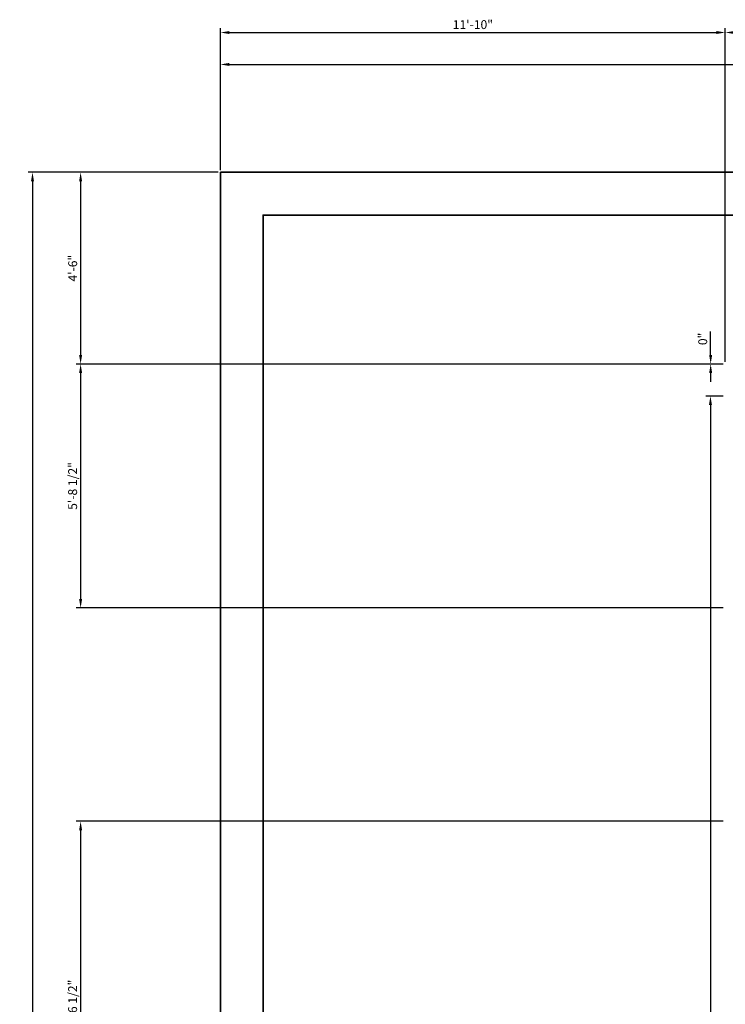
# Model space of a CAD drawing. Units: inches. Extents: x 2901 to 5923, y 918 to 2827.
# Tile 3 of 16: x 4232 to 4430, y 1450 to 1727. Entities that reach past the tile are written whole.
import ezdxf

# ---------------------------------------------------------------- set-up
doc = ezdxf.new("R2010")
doc.units = ezdxf.units.IN
doc.layers.add('A-ANNO-DIMS', color=2, linetype='Continuous', lineweight=18)
doc.layers.add('C-PROP', color=7, linetype='Continuous', lineweight=35)
doc.styles.get("Standard").update_dxf_attribs({"font": 'arial.ttf'})
doc.dimstyles.new('Copy of ISO-25', dxfattribs={"dimtxt": 2.5, "dimasz": 2.5, "dimexe": 1.25, "dimexo": 0.625, "dimtad": 1, "dimdec": 1, "dimlunit": 4, "dimtxsty": 'Standard', "dimcen": 2.5, "dimadec": 0, "dimazin": 0, "dimtfac": 1, "dimtdec": 1, "dimtmove": 0, "dimatfit": 3, "dimfxl": 1, "dimarcsym": 0})

# ---------------------------------------------------------------- blocks, each defined once
blk = doc.blocks.new('*D24')
at = {"layer": 'A-ANNO-DIMS', "color": 0, "lineweight": -2, "transparency": 16777216}
for p, q in [((4287.55, 1684.29), (4234.11, 1684.29)), ((4235.36, 1681.79), (4235.36, 960.79)), ((4287.55, 958.29), (4234.11, 958.29))]:
    blk.add_line(p, q, dxfattribs=at)
at = {"layer": 'A-ANNO-DIMS', "color": 0, "transparency": 16777216}
for points in [[(4234.95, 1681.79), (4235.78, 1681.79), (4235.36, 1684.29)], [(4234.95, 960.79), (4235.78, 960.79), (4235.36, 958.29)]]:
    blk.add_solid(points, dxfattribs=at)
at = {"layer": 'Defpoints', "color": 0, "transparency": 16777216}
for p in [(4288.18, 1684.29), (4235.36, 958.29), (4288.18, 958.29)]:
    blk.add_point(p, dxfattribs=at)
at = {"layer": 'A-ANNO-DIMS', "color": 0, "transparency": 16777216, "insert": (4233.46, 1321.29), "char_height": 2.5, "attachment_point": 5, "rotation": 90}
blk.add_mtext('60\'-6"', dxfattribs=at)
blk = doc.blocks.new('*D25')
at = {"layer": 'A-ANNO-DIMS', "color": 0, "lineweight": -2, "transparency": 16777216}
for p, q in [((4288.18, 1684.92), (4288.18, 1715.87)), ((4290.68, 1714.62), (5012.68, 1714.62)), ((5015.18, 1684.92), (5015.18, 1715.87))]:
    blk.add_line(p, q, dxfattribs=at)
at = {"layer": 'A-ANNO-DIMS', "color": 0, "transparency": 16777216}
for points in [[(4290.68, 1715.04), (4290.68, 1714.2), (4288.18, 1714.62)], [(5012.68, 1715.04), (5012.68, 1714.2), (5015.18, 1714.62)]]:
    blk.add_solid(points, dxfattribs=at)
at = {"layer": 'Defpoints', "color": 0, "transparency": 16777216}
for p in [(5015.18, 1714.62), (4288.18, 1684.29), (5015.18, 1684.29)]:
    blk.add_point(p, dxfattribs=at)
at = {"layer": 'A-ANNO-DIMS', "color": 0, "transparency": 16777216, "insert": (4651.68, 1716.52), "char_height": 2.5, "attachment_point": 5}
blk.add_mtext('60\'-7"', dxfattribs=at)
blk = doc.blocks.new('*D26')
at = {"layer": 'A-ANNO-DIMS', "color": 0, "lineweight": -2, "transparency": 16777216}
for p, q in [((4425.95, 1632.9), (4425.95, 1639.52)), ((4429.44, 1630.4), (4424.7, 1630.4)), ((4429.44, 1630.4), (4424.7, 1630.4)), ((4425.95, 1627.9), (4425.95, 1625.4))]:
    blk.add_line(p, q, dxfattribs=at)
at = {"layer": 'A-ANNO-DIMS', "color": 0, "transparency": 16777216}
for points in [[(4425.54, 1632.9), (4426.37, 1632.9), (4425.95, 1630.4)], [(4425.54, 1627.9), (4426.37, 1627.9), (4425.95, 1630.4)]]:
    blk.add_solid(points, dxfattribs=at)
at = {"layer": 'Defpoints', "color": 0, "transparency": 16777216}
for p in [(4425.95, 1630.4), (4430.07, 1630.4), (4430.07, 1630.4)]:
    blk.add_point(p, dxfattribs=at)
at = {"layer": 'A-ANNO-DIMS', "color": 0, "transparency": 16777216, "insert": (4424.05, 1637.46), "char_height": 2.5, "attachment_point": 5, "rotation": 90}
blk.add_mtext('0"', dxfattribs=at)
blk = doc.blocks.new('*D27')
at = {"layer": 'A-ANNO-DIMS', "color": 0, "lineweight": -2, "transparency": 16777216}
for p, q in [((4429.44, 1621.4), (4424.64, 1621.4)), ((4425.89, 1618.9), (4425.89, 1248.9)), ((4429.44, 1246.4), (4424.64, 1246.4))]:
    blk.add_line(p, q, dxfattribs=at)
at = {"layer": 'A-ANNO-DIMS', "color": 0, "transparency": 16777216}
for points in [[(4425.47, 1618.9), (4426.31, 1618.9), (4425.89, 1621.4)], [(4425.47, 1248.9), (4426.31, 1248.9), (4425.89, 1246.4)]]:
    blk.add_solid(points, dxfattribs=at)
at = {"layer": 'Defpoints', "color": 0, "transparency": 16777216}
for p in [(4430.07, 1621.4), (4425.89, 1246.4), (4430.07, 1246.4)]:
    blk.add_point(p, dxfattribs=at)
at = {"layer": 'A-ANNO-DIMS', "color": 0, "transparency": 16777216, "insert": (4423.99, 1433.9), "char_height": 2.5, "attachment_point": 5, "rotation": 90}
blk.add_mtext('31\'-3"', dxfattribs=at)
blk = doc.blocks.new('*D90')
at = {"layer": 'A-ANNO-DIMS', "color": 0, "lineweight": -2, "transparency": 16777216}
for p, q in [((4288.18, 1684.92), (4288.18, 1724.84)), ((4430.07, 1631.02), (4430.07, 1724.84)), ((4290.68, 1723.59), (4427.57, 1723.59))]:
    blk.add_line(p, q, dxfattribs=at)
at = {"layer": 'A-ANNO-DIMS', "color": 0, "transparency": 16777216}
for points in [[(4290.68, 1724.01), (4290.68, 1723.18), (4288.18, 1723.59)], [(4427.57, 1724.01), (4427.57, 1723.18), (4430.07, 1723.59)]]:
    blk.add_solid(points, dxfattribs=at)
at = {"layer": 'Defpoints', "color": 0, "transparency": 16777216}
for p in [(4430.07, 1723.59), (4288.18, 1684.29), (4430.07, 1630.4)]:
    blk.add_point(p, dxfattribs=at)
at = {"layer": 'A-ANNO-DIMS', "color": 0, "transparency": 16777216, "insert": (4359.12, 1725.49), "char_height": 2.5, "attachment_point": 5}
blk.add_mtext('11\'-10"', dxfattribs=at)
blk = doc.blocks.new('*D91')
at = {"layer": 'A-ANNO-DIMS', "color": 0, "lineweight": -2, "transparency": 16777216}
for p, q in [((4287.55, 1684.29), (4247.63, 1684.29)), ((4248.88, 1681.79), (4248.88, 1632.9)), ((4429.44, 1630.4), (4247.63, 1630.4))]:
    blk.add_line(p, q, dxfattribs=at)
at = {"layer": 'A-ANNO-DIMS', "color": 0, "transparency": 16777216}
for points in [[(4248.46, 1681.79), (4249.3, 1681.79), (4248.88, 1684.29)], [(4248.46, 1632.9), (4249.3, 1632.9), (4248.88, 1630.4)]]:
    blk.add_solid(points, dxfattribs=at)
at = {"layer": 'Defpoints', "color": 0, "transparency": 16777216}
for p in [(4288.18, 1684.29), (4248.88, 1630.4), (4430.07, 1630.4)]:
    blk.add_point(p, dxfattribs=at)
at = {"layer": 'A-ANNO-DIMS', "color": 0, "transparency": 16777216, "insert": (4246.98, 1657.34), "char_height": 2.5, "attachment_point": 5, "rotation": 90}
blk.add_mtext('4\'-6"', dxfattribs=at)
blk = doc.blocks.new('*D92')
at = {"layer": 'A-ANNO-DIMS', "color": 0, "lineweight": -2, "transparency": 16777216}
for p, q in [((4430.07, 1631.02), (4430.07, 1724.84)), ((4487.07, 1631.02), (4487.07, 1724.84)), ((4432.57, 1723.59), (4484.57, 1723.59))]:
    blk.add_line(p, q, dxfattribs=at)
at = {"layer": 'A-ANNO-DIMS', "color": 0, "transparency": 16777216}
for points in [[(4432.57, 1724.01), (4432.57, 1723.18), (4430.07, 1723.59)], [(4484.57, 1724.01), (4484.57, 1723.18), (4487.07, 1723.59)]]:
    blk.add_solid(points, dxfattribs=at)
at = {"layer": 'Defpoints', "color": 0, "transparency": 16777216}
for p in [(4487.07, 1723.59), (4430.07, 1630.4), (4487.07, 1630.4)]:
    blk.add_point(p, dxfattribs=at)
at = {"layer": 'A-ANNO-DIMS', "color": 0, "transparency": 16777216, "insert": (4458.57, 1725.49), "char_height": 2.5, "attachment_point": 5}
blk.add_mtext('4\'-9"', dxfattribs=at)
blk = doc.blocks.new('*D94')
at = {"layer": 'A-ANNO-DIMS', "color": 0, "lineweight": -2, "transparency": 16777216}
for p, q in [((4429.44, 1630.4), (4247.63, 1630.4)), ((4248.88, 1627.9), (4248.88, 1564.34)), ((4429.44, 1561.84), (4247.63, 1561.84))]:
    blk.add_line(p, q, dxfattribs=at)
at = {"layer": 'A-ANNO-DIMS', "color": 0, "transparency": 16777216}
for points in [[(4248.46, 1627.9), (4249.3, 1627.9), (4248.88, 1630.4)], [(4248.46, 1564.34), (4249.3, 1564.34), (4248.88, 1561.84)]]:
    blk.add_solid(points, dxfattribs=at)
at = {"layer": 'Defpoints', "color": 0, "transparency": 16777216}
for p in [(4430.07, 1630.4), (4248.88, 1561.84), (4430.07, 1561.84)]:
    blk.add_point(p, dxfattribs=at)
at = {"layer": 'A-ANNO-DIMS', "color": 0, "transparency": 16777216, "insert": (4246.96, 1596.12), "char_height": 2.5, "attachment_point": 5, "rotation": 90}
blk.add_mtext('5\'-8 1/2"', dxfattribs=at)
blk = doc.blocks.new('*D95')
at = {"layer": 'A-ANNO-DIMS', "color": 0, "lineweight": -2, "transparency": 16777216}
for p, q in [((4429.44, 1501.84), (4247.63, 1501.84)), ((4248.88, 1499.34), (4248.88, 1401.9)), ((4429.44, 1399.4), (4247.63, 1399.4))]:
    blk.add_line(p, q, dxfattribs=at)
at = {"layer": 'A-ANNO-DIMS', "color": 0, "transparency": 16777216}
for points in [[(4248.46, 1499.34), (4249.3, 1499.34), (4248.88, 1501.84)], [(4248.46, 1401.9), (4249.3, 1401.9), (4248.88, 1399.4)]]:
    blk.add_solid(points, dxfattribs=at)
at = {"layer": 'Defpoints', "color": 0, "transparency": 16777216}
for p in [(4430.07, 1501.84), (4248.88, 1399.4), (4430.07, 1399.4)]:
    blk.add_point(p, dxfattribs=at)
at = {"layer": 'A-ANNO-DIMS', "color": 0, "transparency": 16777216, "insert": (4246.96, 1450.62), "char_height": 2.5, "attachment_point": 5, "rotation": 90}
blk.add_mtext('8\'-6 1/2"', dxfattribs=at)

msp = doc.modelspace()

# ---------------------------------------------------------------- linework, layer by layer
at = {"layer": 'C-PROP'}
msp.add_lwpolyline([(4288.18, 1684.29), (5015.18, 1684.29), (5015.18, 958.29), (4288.18, 958.29)], close=True, dxfattribs=at)
msp.add_lwpolyline([(5003.18, 978.26), (5003.18, 970.29), (4300.18, 970.29), (4300.18, 1672.29), (5003.18, 1672.29), (5003.18, 1132.27)], dxfattribs=at)

# ---------------------------------------------------------------- dimensions: what is measured, and where the dimension line sits
at = {"layer": 'A-ANNO-DIMS'}
for base, p1, p2, override, picture, middle in [((4430.07, 1723.59), (4288.18, 1684.29), (4430.07, 1630.4), {"dimdec": 1, "dimlfac": 1, "dimrnd": 0, "dimzin": 1, "dimdsep": 46, "dimlunit": 4, "dimfrac": 2}, '*D90', (4359.12, 1725.49)), ((4487.07, 1723.59), (4430.07, 1630.4), (4487.07, 1630.4), {"dimdec": 1, "dimlfac": 1, "dimrnd": 0, "dimzin": 1, "dimdsep": 46, "dimlunit": 4, "dimfrac": 2}, '*D92', (4458.57, 1725.49)), ((5015.18, 1714.62), (4288.18, 1684.29), (5015.18, 1684.29), {"dimclrd": 0, "dimclre": 0, "dimclrt": 0}, '*D25', (4651.68, 1716.52))]:
    dim = msp.add_linear_dim(base=base, p1=p1, p2=p2, dimstyle='Copy of ISO-25', override=override, dxfattribs=at)
    dim.commit()
    dim.dimension.update_dxf_attribs({"geometry": picture, "text_midpoint": middle})
for base, p1, p2, override, picture, middle in [((4235.36, 958.29), (4288.18, 1684.29), (4288.18, 958.29), {"dimclrd": 0, "dimclre": 0, "dimclrt": 0}, '*D24', (4233.46, 1321.29)), ((4248.88, 1630.4), (4288.18, 1684.29), (4430.07, 1630.4), {"dimdec": 1, "dimlfac": 1, "dimrnd": 0, "dimzin": 1, "dimdsep": 46, "dimlunit": 4, "dimfrac": 2}, '*D91', (4246.98, 1657.34)), ((4425.95179115, 1630.39662355), (4430.0684223, 1630.39662355), (4430.0684223, 1630.39662355), {"dimclrd": 0, "dimclre": 0, "dimclrt": 0}, '*D26', (4424.05035868, 1637.45835615)), ((4248.88, 1561.84), (4430.07, 1630.4), (4430.07, 1561.84), {"dimdec": 1, "dimlfac": 1, "dimrnd": 0, "dimzin": 1, "dimdsep": 46, "dimlunit": 4, "dimfrac": 2}, '*D94', (4246.96, 1596.12)), ((4425.89, 1246.4), (4430.07, 1621.4), (4430.07, 1246.4), {"dimclrd": 0, "dimclre": 0, "dimclrt": 0}, '*D27', (4423.99, 1433.9)), ((4248.88, 1399.4), (4430.07, 1501.84), (4430.07, 1399.4), {"dimdec": 1, "dimlfac": 1, "dimrnd": 0, "dimzin": 1, "dimdsep": 46, "dimlunit": 4, "dimfrac": 2}, '*D95', (4246.96, 1450.62))]:
    dim = msp.add_linear_dim(base=base, p1=p1, p2=p2, angle=90, dimstyle='Copy of ISO-25', override=override, dxfattribs=at)
    dim.commit()
    dim.dimension.update_dxf_attribs({"geometry": picture, "text_midpoint": middle})

doc.saveas('drawing.dxf')
